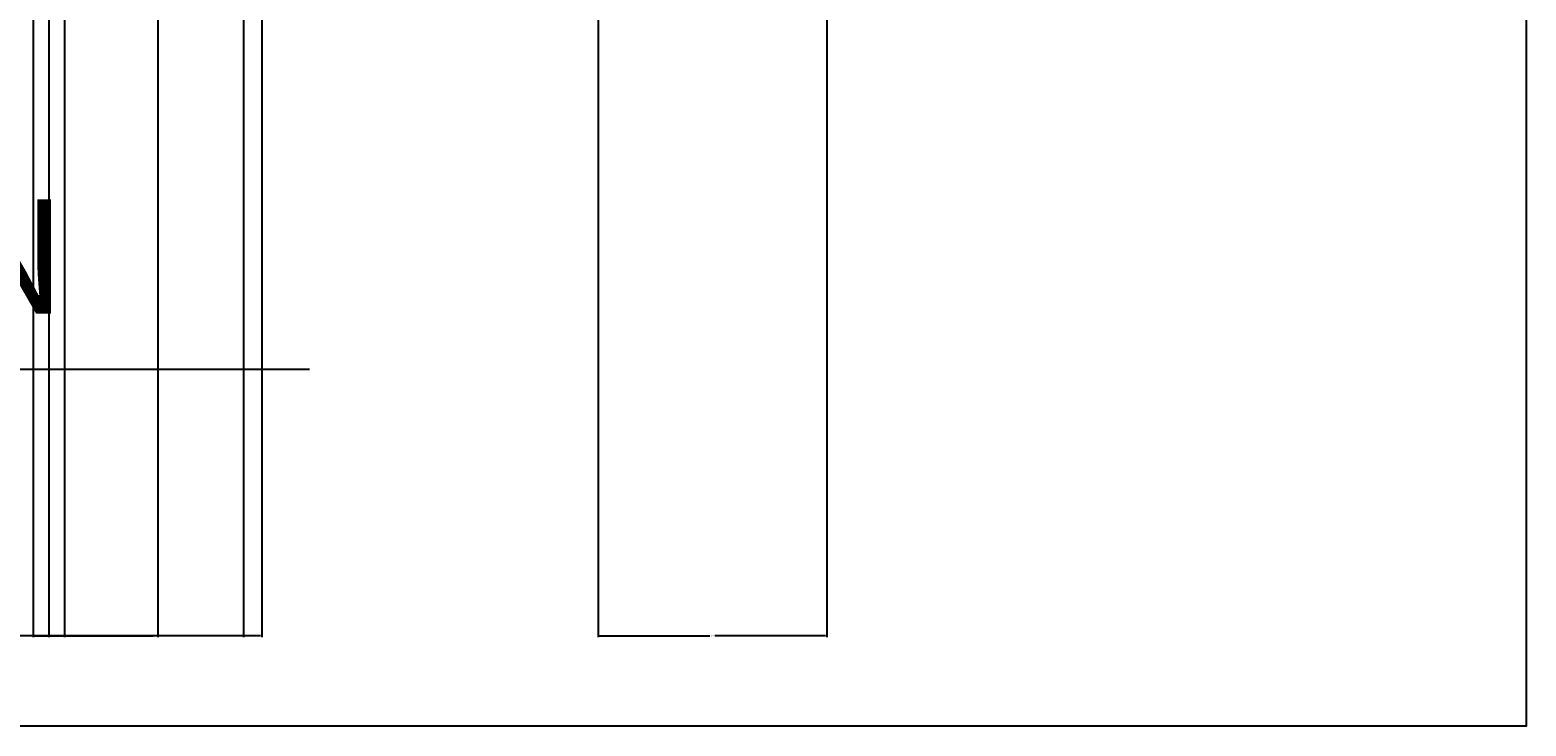
# Model space of a CAD drawing. Units: inches. Extents: x 1748 to 2382, y 1346 to 2284.
# Tile 12 of 26: x 2147 to 2382, y 1346 to 1456. Entities that reach past the tile are written whole.
import ezdxf

# ---------------------------------------------------------------- set-up
doc = ezdxf.new("R2010")
doc.units = ezdxf.units.IN
for name, color, linetype, lineweight in [('A-ANNO-DIMS', 2, 'Continuous', 18), ('A-ANNO-TTLB', 7, 'Continuous', 25), ('A-WALL-PATT', 9, 'Continuous', 13)]:
    doc.layers.add(name, color=color, linetype=linetype, lineweight=lineweight)
doc.styles.get("Standard").update_dxf_attribs({"font": 'arial.ttf'})
doc.dimstyles.get("Standard").update_dxf_attribs({"dimtxt": 0.18, "dimasz": 0.18, "dimexe": 0.18, "dimexo": 0.0625, "dimgap": 0.09, "dimtad": 0, "dimtih": 1, "dimtoh": 1, "dimdec": 4, "dimzin": 0, "dimdsep": 46, "dimtxsty": 'Standard', "dimcen": 0.09, "dimadec": 0, "dimazin": 0, "dimtfac": 1, "dimtdec": 4, "dimtofl": 0, "dimtmove": 0, "dimatfit": 3, "dimfxl": 1, "dimtolj": 1, "dimtzin": 0, "dimarcsym": 0})

# ---------------------------------------------------------------- blocks, each defined once
blk = doc.blocks.new('*D46')
at = {"layer": 'A-ANNO-DIMS', "color": 0, "lineweight": -2, "transparency": 16777216}
for p, q in [((2147.39, 1725.79), (2147.39, 1360.47)), ((2180.46, 1725.79), (2180.46, 1360.47)), ((2147.57, 1360.65), (2163.46, 1360.65)), ((2180.28, 1360.65), (2164.39, 1360.65))]:
    blk.add_line(p, q, dxfattribs=at)
at = {"layer": 'A-ANNO-DIMS', "color": 0, "transparency": 16777216}
for points in [[(2147.57, 1360.68), (2147.57, 1360.62), (2147.39, 1360.65)], [(2180.28, 1360.68), (2180.28, 1360.62), (2180.46, 1360.65)]]:
    blk.add_solid(points, dxfattribs=at)
at = {"layer": 'Defpoints', "color": 0, "transparency": 16777216}
for p in [(2147.39, 1725.85), (2180.46, 1725.85), (2180.46, 1360.65)]:
    blk.add_point(p, dxfattribs=at)
at = {"layer": 'A-ANNO-DIMS', "color": 0, "transparency": 16777216, "insert": (2163.92, 1360.65), "char_height": 0.18, "attachment_point": 5}
blk.add_mtext('\\A1;33.066', dxfattribs=at)
blk = doc.blocks.new('*D47')
at = {"layer": 'A-ANNO-DIMS', "color": 0, "lineweight": -2, "transparency": 16777216}
for p, q in [((2149.85, 1913.29), (2149.85, 1360.47)), ((2183.35, 1913.29), (2183.35, 1360.47)), ((2150.03, 1360.65), (2166.28, 1360.65)), ((2183.17, 1360.65), (2166.93, 1360.65))]:
    blk.add_line(p, q, dxfattribs=at)
at = {"layer": 'A-ANNO-DIMS', "color": 0, "transparency": 16777216}
for points in [[(2150.03, 1360.68), (2150.03, 1360.62), (2149.85, 1360.65)], [(2183.17, 1360.68), (2183.17, 1360.62), (2183.35, 1360.65)]]:
    blk.add_solid(points, dxfattribs=at)
at = {"layer": 'Defpoints', "color": 0, "transparency": 16777216}
for p in [(2149.85, 1913.35), (2183.35, 1913.35), (2183.35, 1360.65)]:
    blk.add_point(p, dxfattribs=at)
at = {"layer": 'A-ANNO-DIMS', "color": 0, "transparency": 16777216, "insert": (2166.6, 1360.65), "char_height": 0.18, "attachment_point": 5}
blk.add_mtext('\\A1;33.5', dxfattribs=at)
blk = doc.blocks.new('*D49')
at = {"layer": 'A-ANNO-DIMS', "color": 0, "lineweight": -2, "transparency": 16777216}
for p, q in [((2236.23, 1913.29), (2236.23, 1360.47)), ((2272.19, 1913.29), (2272.19, 1360.47)), ((2236.41, 1360.65), (2253.82, 1360.65)), ((2272.01, 1360.65), (2254.61, 1360.65))]:
    blk.add_line(p, q, dxfattribs=at)
at = {"layer": 'A-ANNO-DIMS', "color": 0, "transparency": 16777216}
for points in [[(2236.41, 1360.68), (2236.41, 1360.62), (2236.23, 1360.65)], [(2272.01, 1360.68), (2272.01, 1360.62), (2272.19, 1360.65)]]:
    blk.add_solid(points, dxfattribs=at)
at = {"layer": 'Defpoints', "color": 0, "transparency": 16777216}
for p in [(2236.23, 1913.35), (2272.19, 1913.35), (2272.19, 1360.65)]:
    blk.add_point(p, dxfattribs=at)
at = {"layer": 'A-ANNO-DIMS', "color": 0, "transparency": 16777216, "insert": (2254.21, 1360.65), "char_height": 0.18, "attachment_point": 5}
blk.add_mtext('\\A1;35.96', dxfattribs=at)
blk = doc.blocks.new('*D53')
at = {"layer": 'A-ANNO-DIMS', "color": 0, "lineweight": -2, "transparency": 16777216}
for p, q in [((2115.4, 2223.79), (2115.4, 1360.47)), ((2167.02, 2223.79), (2167.02, 1360.47)), ((2115.58, 1360.65), (2140.81, 1360.65)), ((2166.84, 1360.65), (2141.6, 1360.65))]:
    blk.add_line(p, q, dxfattribs=at)
at = {"layer": 'A-ANNO-DIMS', "color": 0, "transparency": 16777216}
for points in [[(2115.58, 1360.68), (2115.58, 1360.62), (2115.4, 1360.65)], [(2166.84, 1360.68), (2166.84, 1360.62), (2167.02, 1360.65)]]:
    blk.add_solid(points, dxfattribs=at)
at = {"layer": 'Defpoints', "color": 0, "transparency": 16777216}
for p in [(2115.4, 2223.85), (2167.02, 2223.85), (2167.02, 1360.65)]:
    blk.add_point(p, dxfattribs=at)
at = {"layer": 'A-ANNO-DIMS', "color": 0, "transparency": 16777216, "insert": (2141.21, 1360.65), "char_height": 0.18, "attachment_point": 5}
blk.add_mtext('\\A1;51.62', dxfattribs=at)
blk = doc.blocks.new('*D67')
at = {"layer": 'A-ANNO-DIMS', "color": 0, "lineweight": -2, "transparency": 16777216}
for p, q in [((2095.36, 1467.79), (2095.36, 1360.47)), ((2152.34, 1467.79), (2152.34, 1360.47)), ((2095.54, 1360.65), (2123.45, 1360.65)), ((2152.16, 1360.65), (2124.24, 1360.65))]:
    blk.add_line(p, q, dxfattribs=at)
at = {"layer": 'A-ANNO-DIMS', "color": 0, "transparency": 16777216}
for points in [[(2095.54, 1360.68), (2095.54, 1360.62), (2095.36, 1360.65)], [(2152.16, 1360.68), (2152.16, 1360.62), (2152.34, 1360.65)]]:
    blk.add_solid(points, dxfattribs=at)
at = {"layer": 'Defpoints', "color": 0, "transparency": 16777216}
for p in [(2095.36, 1467.85), (2152.34, 1467.85), (2152.34, 1360.65)]:
    blk.add_point(p, dxfattribs=at)
at = {"layer": 'A-ANNO-DIMS', "color": 0, "transparency": 16777216, "insert": (2123.85, 1360.65), "char_height": 0.18, "attachment_point": 5}
blk.add_mtext('\\A1;56.97', dxfattribs=at)

msp = doc.modelspace()

# ---------------------------------------------------------------- hatches: boundary and pattern name
at = {"layer": 'A-WALL-PATT'}
h = msp.add_hatch(dxfattribs=at)
h.set_pattern_fill('ANSI32', color=256)
h.paths.add_polyline_path([(1908.4445, 2232.8497), (1821.9607, 2232.8497), (1821.9607, 2223.8497), (1865.4607, 2223.8497), (1865.4607, 2209.9185), (1869.9607, 2209.9185), (1869.9607, 2223.8497), (1908.4445, 2223.8497), (1908.4445, 2228.3497)])
h.paths.add_polyline_path([(2040.0683, 2232.8497), (1968.4445, 2232.8497), (1968.4445, 2223.8497), (2025.9607, 2223.8497), (2025.9607, 2130.3497), (2032.1341, 2130.3497), (2032.1341, 2132.5997), (2032.1341, 2134.8497), (2030.4607, 2134.8497), (2030.4607, 2223.8497), (2040.0683, 2223.8497)])
h.paths.add_polyline_path([(2091.3969, 2232.8497), (2064.0683, 2232.8497), (2064.0683, 2223.8497), (2078.4607, 2223.8497), (2078.4607, 2134.8497), (2051.1563, 2134.8497), (2051.1563, 2130.3497), (2078.4607, 2130.3497), (2078.4607, 2128.6813), (2082.9607, 2128.6813), (2082.9607, 2130.3497), (2086.1879, 2130.3497), (2086.1879, 2132.5997), (2086.1879, 2134.8497), (2082.9607, 2134.8497), (2082.9607, 2223.8497), (2091.3969, 2223.8497), (2091.3969, 2228.3497)])
h.paths.add_polyline_path([(2167.0164, 2232.8497), (2115.3969, 2232.8497), (2115.3969, 2223.8497), (2130.9607, 2223.8497), (2130.9607, 2134.8497), (2106.9607, 2134.8497), (2106.9607, 2130.3497), (2135.4607, 2130.3497), (2135.4607, 2223.8497), (2167.0164, 2223.8497), (2167.0164, 2228.3497)])
h.paths.add_polyline_path([(1869.9607, 2149.9185), (1865.4607, 2149.9185), (1865.4607, 2127.8942), (1869.9607, 2127.8942)])
h.paths.add_polyline_path([(2082.9607, 2104.4871), (2080.7107, 2104.4871), (2078.4607, 2104.4871), (2078.4607, 2103.8497), (1869.9607, 2103.8497), (1869.9607, 2108.6062), (1867.7107, 2108.6062), (1865.4607, 2108.6062), (1865.4607, 2103.8497), (1821.9607, 2103.8497), (1821.9607, 2099.3497), (1865.4607, 2099.3497), (1865.4607, 2094.7509), (1869.9607, 2094.7509), (1869.9607, 2099.3497), (2025.9607, 2099.3497), (2025.9607, 2096.4326), (2030.4607, 2096.4326), (2030.4607, 2099.3497), (2082.9607, 2099.3497)])
h.paths.add_polyline_path([(1928.9457, 1401.1212), (2176.8693, 1401.1212), (2176.8693, 1438.214), (1928.9457, 1438.214)], flags=9)
h.paths.add_polyline_path([(2122.2668, 2048.1927), (2177.9387, 2048.1927), (2177.9387, 2066.85), (2122.2668, 2066.85)], flags=9)
h.paths.add_polyline_path([(2272.688, 2153.8197), (2272.688, 2216.746), (2262.3845, 2216.746), (2262.3845, 2153.8197)], flags=9)
h.paths.add_polyline_path([(2157.2928, 2166.5593), (2196.3822, 2166.5593), (2196.3822, 2185.2167), (2157.2928, 2185.2167)], flags=9)
h.paths.add_polyline_path([(2089.3407, 2162.0698), (2124.3987, 2162.0698), (2124.3987, 2180.7272), (2089.3407, 2180.7272)], flags=9)
h.paths.add_polyline_path([(2037.4521, 2160.0913), (2072.5101, 2160.0913), (2072.5101, 2178.7486), (2037.4521, 2178.7486)], flags=9)
h.paths.add_polyline_path([(1884.7894, 2104.1554), (1923.6297, 2104.1554), (1923.6297, 2122.8127), (1884.7894, 2122.8127)], flags=9)
h.paths.add_polyline_path([(1851.2832, 2142.9749), (1851.2832, 2199.3051), (1840.9796, 2199.3051), (1840.9796, 2142.9749)], flags=9)
h.paths.add_polyline_path([(1844.8763, 2017.2834), (1844.8763, 2073.6136), (1834.5728, 2073.6136), (1834.5728, 2017.2834)], flags=9)
h.paths.add_polyline_path([(1897.1577, 2073.1279), (1935.9981, 2073.1279), (1935.9981, 2091.7853), (1897.1577, 2091.7853)], flags=9)
h.paths.add_polyline_path([(1952.3395, 1802.4231), (2008.0114, 1802.4231), (2008.0114, 1821.0805), (1952.3395, 1821.0805)], flags=9)
h.paths.add_polyline_path([(1978.8184, 1857.6841), (2017.7338, 1857.6841), (2017.7338, 1876.3415), (1978.8184, 1876.3415)], flags=9)
h.paths.add_polyline_path([(1979.6513, 1925.9516), (2008.8089, 1925.9516), (2008.8089, 1944.6089), (1979.6513, 1944.6089)], flags=9)
h.paths.add_polyline_path([(1838.5553, 1860.3527), (1877.3957, 1860.3527), (1877.3957, 1879.01), (1838.5553, 1879.01)], flags=9)
h.paths.add_polyline_path([(1883.9018, 1787.3013), (1883.9018, 1843.6315), (1873.5983, 1843.6315), (1873.5983, 1787.3013)], flags=9)
h.paths.add_polyline_path([(1873.7079, 1509.1938), (1873.7079, 1583.7709), (1863.4044, 1583.7709), (1863.4044, 1509.1938)], flags=9)
h.paths.add_polyline_path([(1916.2259, 1603.3681), (1955.0663, 1603.3681), (1955.0663, 1622.0254), (1916.2259, 1622.0254)], flags=9)
h.paths.add_polyline_path([(1876.3013, 1636.757), (1876.3013, 1693.0871), (1865.9978, 1693.0871), (1865.9978, 1636.757)], flags=9)
h.paths.add_polyline_path([(1921.3138, 1521.8316), (1964.0662, 1521.8316), (1964.0662, 1540.489), (1921.3138, 1540.489)], flags=9)
h.paths.add_polyline_path([(2017.5657, 1497.5078), (2046.7983, 1497.5078), (2046.7983, 1516.1651), (2017.5657, 1516.1651)], flags=9)
h.paths.add_polyline_path([(2066.8661, 1499.3902), (2096.0988, 1499.3902), (2096.0988, 1518.0475), (2066.8661, 1518.0475)], flags=9)
h.paths.add_polyline_path([(2155.4835, 1571.6596), (2198.2358, 1571.6596), (2198.2358, 1590.3169), (2155.4835, 1590.3169)], flags=9)
h.paths.add_polyline_path([(2094.9136, 1664.6812), (2150.5855, 1664.6812), (2150.5855, 1683.3386), (2094.9136, 1683.3386)], flags=9)
h.paths.add_polyline_path([(2257.6902, 1863.1628), (2269.8935, 1863.1628), (2269.8935, 1873.4664), (2257.6902, 1873.4664)], flags=9)
h.paths.add_polyline_path([(2164.0748, 1880.3089), (2189.8694, 1880.3089), (2189.8694, 1890.6124), (2164.0748, 1890.6124)], flags=9)
h.paths.add_polyline_path([(2239.4394, 1931.0585), (2268.8187, 1931.0585), (2268.8187, 1949.7159), (2239.4394, 1949.7159)], flags=9)
h = msp.add_hatch(dxfattribs=at)
h.set_pattern_fill('ANSI32', color=256)
h.paths.add_polyline_path([(2297.4607, 2232.8497), (2203.0164, 2232.8497), (2203.0164, 2223.8497), (2244.9607, 2223.8497), (2244.9607, 2127.8554), (2249.4607, 2127.8554), (2249.4607, 2223.8497), (2297.4607, 2223.8497)])
h.paths.add_polyline_path([(2297.4607, 2103.8497), (2249.4607, 2103.8497), (2249.4607, 2106.7497), (2247.2107, 2106.7497), (2244.9607, 2106.7497), (2244.9607, 2103.8497), (2130.9607, 2103.8497), (2130.9607, 2099.3497), (2288.4607, 2099.3497), (2288.4607, 2077.2008), (2297.4607, 2077.2008)])
h.paths.add_polyline_path([(1928.9457, 1401.1212), (2176.8693, 1401.1212), (2176.8693, 1438.214), (1928.9457, 1438.214)], flags=9)
h.paths.add_polyline_path([(2122.2668, 2048.1927), (2177.9387, 2048.1927), (2177.9387, 2066.85), (2122.2668, 2066.85)], flags=9)
h.paths.add_polyline_path([(2272.688, 2153.8197), (2272.688, 2216.746), (2262.3845, 2216.746), (2262.3845, 2153.8197)], flags=25)
h.paths.add_polyline_path([(2157.2928, 2166.5593), (2196.3822, 2166.5593), (2196.3822, 2185.2167), (2157.2928, 2185.2167)], flags=9)
h.paths.add_polyline_path([(2089.3407, 2162.0698), (2124.3987, 2162.0698), (2124.3987, 2180.7272), (2089.3407, 2180.7272)], flags=9)
h.paths.add_polyline_path([(2037.4521, 2160.0913), (2072.5101, 2160.0913), (2072.5101, 2178.7486), (2037.4521, 2178.7486)], flags=9)
h.paths.add_polyline_path([(1884.7894, 2104.1554), (1923.6297, 2104.1554), (1923.6297, 2122.8127), (1884.7894, 2122.8127)], flags=9)
h.paths.add_polyline_path([(1851.2832, 2142.9749), (1851.2832, 2199.3051), (1840.9796, 2199.3051), (1840.9796, 2142.9749)], flags=9)
h.paths.add_polyline_path([(1844.8763, 2017.2834), (1844.8763, 2073.6136), (1834.5728, 2073.6136), (1834.5728, 2017.2834)], flags=9)
h.paths.add_polyline_path([(1897.1577, 2073.1279), (1935.9981, 2073.1279), (1935.9981, 2091.7853), (1897.1577, 2091.7853)], flags=9)
h.paths.add_polyline_path([(1952.3395, 1802.4231), (2008.0114, 1802.4231), (2008.0114, 1821.0805), (1952.3395, 1821.0805)], flags=9)
h.paths.add_polyline_path([(1978.8184, 1857.6841), (2017.7338, 1857.6841), (2017.7338, 1876.3415), (1978.8184, 1876.3415)], flags=9)
h.paths.add_polyline_path([(1979.6513, 1925.9516), (2008.8089, 1925.9516), (2008.8089, 1944.6089), (1979.6513, 1944.6089)], flags=9)
h.paths.add_polyline_path([(1838.5553, 1860.3527), (1877.3957, 1860.3527), (1877.3957, 1879.01), (1838.5553, 1879.01)], flags=9)
h.paths.add_polyline_path([(1883.9018, 1787.3013), (1883.9018, 1843.6315), (1873.5983, 1843.6315), (1873.5983, 1787.3013)], flags=9)
h.paths.add_polyline_path([(1873.7079, 1509.1938), (1873.7079, 1583.7709), (1863.4044, 1583.7709), (1863.4044, 1509.1938)], flags=9)
h.paths.add_polyline_path([(1916.2259, 1603.3681), (1955.0663, 1603.3681), (1955.0663, 1622.0254), (1916.2259, 1622.0254)], flags=9)
h.paths.add_polyline_path([(1876.3013, 1636.757), (1876.3013, 1693.0871), (1865.9978, 1693.0871), (1865.9978, 1636.757)], flags=9)
h.paths.add_polyline_path([(1921.3138, 1521.8316), (1964.0662, 1521.8316), (1964.0662, 1540.489), (1921.3138, 1540.489)], flags=9)
h.paths.add_polyline_path([(2017.5657, 1497.5078), (2046.7983, 1497.5078), (2046.7983, 1516.1651), (2017.5657, 1516.1651)], flags=9)
h.paths.add_polyline_path([(2066.8661, 1499.3902), (2096.0988, 1499.3902), (2096.0988, 1518.0475), (2066.8661, 1518.0475)], flags=9)
h.paths.add_polyline_path([(2155.4835, 1571.6596), (2198.2358, 1571.6596), (2198.2358, 1590.3169), (2155.4835, 1590.3169)], flags=9)
h.paths.add_polyline_path([(2094.9136, 1664.6812), (2150.5855, 1664.6812), (2150.5855, 1683.3386), (2094.9136, 1683.3386)], flags=9)
h.paths.add_polyline_path([(2257.6902, 1863.1628), (2269.8935, 1863.1628), (2269.8935, 1873.4664), (2257.6902, 1873.4664)], flags=9)
h.paths.add_polyline_path([(2164.0748, 1880.3089), (2189.8694, 1880.3089), (2189.8694, 1890.6124), (2164.0748, 1890.6124)], flags=9)
h.paths.add_polyline_path([(2239.4394, 1931.0585), (2268.8187, 1931.0585), (2268.8187, 1949.7159), (2239.4394, 1949.7159)], flags=9)
h = msp.add_hatch(dxfattribs=at)
h.set_pattern_fill('ANSI32', color=256)
h.paths.add_polyline_path([(1919.6777, 1476.8497), (1900.6426, 1476.8497), (1900.6426, 1522.0826), (1898.3926, 1522.0826), (1896.1426, 1522.0826), (1896.1426, 1476.8497), (1857.1426, 1476.8497), (1857.1426, 1467.8497), (1896.1426, 1467.8497), (1919.6777, 1467.8497), (1919.6777, 1472.3497)])
h.paths.add_polyline_path([(2018.7873, 1472.3497), (2018.7873, 1476.8497), (2010.9607, 1476.8497), (2010.9607, 1560.8497), (2034.9607, 1560.8497), (2034.9607, 1565.3497), (2006.4607, 1565.3497), (2006.4607, 1476.8497), (1955.6777, 1476.8497), (1955.6777, 1467.8497), (2018.7873, 1467.8497)])
h.paths.add_polyline_path([(2152.3354, 1472.3497), (2152.3354, 1476.8497), (2115.9607, 1476.8497), (2115.9607, 1565.3497), (2109.2204, 1565.3497), (2109.2204, 1563.0997), (2109.2204, 1560.8497), (2111.4607, 1560.8497), (2111.4607, 1476.8497), (2095.3617, 1476.8497), (2095.3617, 1467.8497), (2152.3354, 1467.8497)])
h.paths.add_polyline_path([(2071.3617, 1476.8497), (2063.4607, 1476.8497), (2063.4607, 1560.8497), (2090.1865, 1560.8497), (2090.1865, 1565.3497), (2063.4607, 1565.3497), (2063.4607, 1572.5485), (2061.2107, 1572.5485), (2058.9607, 1572.5485), (2058.9607, 1565.3497), (2055.6281, 1565.3497), (2055.6281, 1560.8497), (2058.9607, 1560.8497), (2058.9607, 1476.8497), (2042.7873, 1476.8497), (2042.7873, 1467.8497), (2071.3617, 1467.8497), (2071.3617, 1472.3497)])
h.paths.add_polyline_path([(2297.4607, 1506.5652), (2288.4607, 1506.5652), (2288.4607, 1476.8497), (2212.3354, 1476.8497), (2212.3354, 1467.8497), (2297.4607, 1467.8497)])
h.paths.add_polyline_path([(2297.4607, 1645.3038), (2288.4607, 1645.3038), (2288.4607, 1605.8497), (2058.9607, 1605.8497), (2058.9607, 1600.1857), (2061.2107, 1600.1857), (2063.4607, 1600.1857), (2063.4607, 1601.3497), (2288.4607, 1601.3497), (2288.4607, 1566.5652), (2297.4607, 1566.5652)])
h.paths.add_polyline_path([(2010.9607, 1609.0561), (2008.7107, 1609.0561), (2006.4607, 1609.0561), (2006.4607, 1605.8497), (1900.6426, 1605.8497), (1900.6426, 1609.7171), (1898.3926, 1609.7171), (1896.1426, 1609.7171), (1896.1426, 1605.8497), (1857.1426, 1605.8497), (1857.1426, 1601.3497), (1896.1426, 1601.3497), (1896.1426, 1542.5447), (1900.6426, 1542.5447), (1900.6426, 1601.3497), (2010.9607, 1601.3497)])
h.paths.add_polyline_path([(1928.9457, 1401.1212), (2176.8693, 1401.1212), (2176.8693, 1438.214), (1928.9457, 1438.214)], flags=9)
h.paths.add_polyline_path([(2122.2668, 2048.1927), (2177.9387, 2048.1927), (2177.9387, 2066.85), (2122.2668, 2066.85)], flags=9)
h.paths.add_polyline_path([(2272.688, 2153.8197), (2272.688, 2216.746), (2262.3845, 2216.746), (2262.3845, 2153.8197)], flags=9)
h.paths.add_polyline_path([(2157.2928, 2166.5593), (2196.3822, 2166.5593), (2196.3822, 2185.2167), (2157.2928, 2185.2167)], flags=9)
h.paths.add_polyline_path([(2089.3407, 2162.0698), (2124.3987, 2162.0698), (2124.3987, 2180.7272), (2089.3407, 2180.7272)], flags=9)
h.paths.add_polyline_path([(2037.4521, 2160.0913), (2072.5101, 2160.0913), (2072.5101, 2178.7486), (2037.4521, 2178.7486)], flags=9)
h.paths.add_polyline_path([(1884.7894, 2104.1554), (1923.6297, 2104.1554), (1923.6297, 2122.8127), (1884.7894, 2122.8127)], flags=9)
h.paths.add_polyline_path([(1851.2832, 2142.9749), (1851.2832, 2199.3051), (1840.9796, 2199.3051), (1840.9796, 2142.9749)], flags=9)
h.paths.add_polyline_path([(1844.8763, 2017.2834), (1844.8763, 2073.6136), (1834.5728, 2073.6136), (1834.5728, 2017.2834)], flags=9)
h.paths.add_polyline_path([(1897.1577, 2073.1279), (1935.9981, 2073.1279), (1935.9981, 2091.7853), (1897.1577, 2091.7853)], flags=9)
h.paths.add_polyline_path([(1952.3395, 1802.4231), (2008.0114, 1802.4231), (2008.0114, 1821.0805), (1952.3395, 1821.0805)], flags=9)
h.paths.add_polyline_path([(1978.8184, 1857.6841), (2017.7338, 1857.6841), (2017.7338, 1876.3415), (1978.8184, 1876.3415)], flags=9)
h.paths.add_polyline_path([(1979.6513, 1925.9516), (2008.8089, 1925.9516), (2008.8089, 1944.6089), (1979.6513, 1944.6089)], flags=9)
h.paths.add_polyline_path([(1838.5553, 1860.3527), (1877.3957, 1860.3527), (1877.3957, 1879.01), (1838.5553, 1879.01)], flags=9)
h.paths.add_polyline_path([(1883.9018, 1787.3013), (1883.9018, 1843.6315), (1873.5983, 1843.6315), (1873.5983, 1787.3013)], flags=9)
h.paths.add_polyline_path([(1873.7079, 1509.1938), (1873.7079, 1583.7709), (1863.4044, 1583.7709), (1863.4044, 1509.1938)], flags=9)
h.paths.add_polyline_path([(1916.2259, 1603.3681), (1955.0663, 1603.3681), (1955.0663, 1622.0254), (1916.2259, 1622.0254)], flags=9)
h.paths.add_polyline_path([(1876.3013, 1636.757), (1876.3013, 1693.0871), (1865.9978, 1693.0871), (1865.9978, 1636.757)], flags=9)
h.paths.add_polyline_path([(1921.3138, 1521.8316), (1964.0662, 1521.8316), (1964.0662, 1540.489), (1921.3138, 1540.489)], flags=9)
h.paths.add_polyline_path([(2017.5657, 1497.5078), (2046.7983, 1497.5078), (2046.7983, 1516.1651), (2017.5657, 1516.1651)], flags=9)
h.paths.add_polyline_path([(2066.8661, 1499.3902), (2096.0988, 1499.3902), (2096.0988, 1518.0475), (2066.8661, 1518.0475)], flags=9)
h.paths.add_polyline_path([(2155.4835, 1571.6596), (2198.2358, 1571.6596), (2198.2358, 1590.3169), (2155.4835, 1590.3169)], flags=25)
h.paths.add_polyline_path([(2094.9136, 1664.6812), (2150.5855, 1664.6812), (2150.5855, 1683.3386), (2094.9136, 1683.3386)], flags=9)
h.paths.add_polyline_path([(2257.6902, 1863.1628), (2269.8935, 1863.1628), (2269.8935, 1873.4664), (2257.6902, 1873.4664)], flags=9)
h.paths.add_polyline_path([(2164.0748, 1880.3089), (2189.8694, 1880.3089), (2189.8694, 1890.6124), (2164.0748, 1890.6124)], flags=9)
h.paths.add_polyline_path([(2239.4394, 1931.0585), (2268.8187, 1931.0585), (2268.8187, 1949.7159), (2239.4394, 1949.7159)], flags=9)

# ---------------------------------------------------------------- linework, layer by layer
at = {"layer": 'A-ANNO-TTLB'}
msp.add_line((1917.9424, 1402.5451), (2190.8758, 1402.5451), dxfattribs=at)
msp.add_lwpolyline([(1747.8112, 2284.3704), (2382.1361, 2284.3704), (2382.1361, 1346.4899), (1747.8112, 1346.4899)], close=True, dxfattribs=at)

# ---------------------------------------------------------------- texts
at = {"layer": 'A-ANNO-TTLB', "insert": (1935.5085, 1429.2692), "char_height": 18, "attachment_point": 1}
msp.add_mtext_dynamic_manual_height_columns('FIRST FLOOR PLAN', width=709.562865, gutter_width=12.5, heights=[0], dxfattribs=at)

# ---------------------------------------------------------------- dimensions: what is measured, and where the dimension line sits
at = {"layer": 'A-ANNO-DIMS'}
for base, p1, p2, override, picture, middle in [((2167.0164, 1360.6451), (2115.3969, 2223.8497), (2167.0164, 2223.8497), {"dimdec": 2, "dimlfac": 1, "dimrnd": 0, "dimzin": 0, "dimdsep": 46, "dimlunit": 2}, '*D53', (2141.2066, 1360.6451)), ((2183.3516, 1360.6451), (2149.8497, 1913.3497), (2183.3516, 1913.3497), {"dimdec": 1, "dimlfac": 1, "dimrnd": 0, "dimzin": 0, "dimdsep": 46, "dimlunit": 2}, '*D47', (2166.6006, 1360.6451)), ((2272.1921, 1360.6451), (2236.234, 1913.3497), (2272.1921, 1913.3497), {"dimdec": 2, "dimlfac": 1, "dimrnd": 0, "dimzin": 0, "dimdsep": 46, "dimlunit": 2}, '*D49', (2254.213, 1360.6451)), ((2180.4551, 1360.6451), (2147.389, 1725.8497), (2180.4551, 1725.8497), {"dimdec": 3, "dimlfac": 1, "dimrnd": 0, "dimzin": 0, "dimdsep": 46, "dimlunit": 2}, '*D46', (2163.9221, 1360.6451)), ((2152.3354, 1360.6451), (2095.3617, 1467.8497), (2152.3354, 1467.8497), {"dimdec": 2, "dimlfac": 1, "dimrnd": 0, "dimzin": 0, "dimdsep": 46, "dimlunit": 2}, '*D67', (2123.8486, 1360.6451))]:
    dim = msp.add_linear_dim(base=base, p1=p1, p2=p2, dimstyle='Standard', override=override, dxfattribs=at)
    dim.commit()
    dim.dimension.update_dxf_attribs({"geometry": picture, "text_midpoint": middle})

doc.saveas('drawing.dxf')
